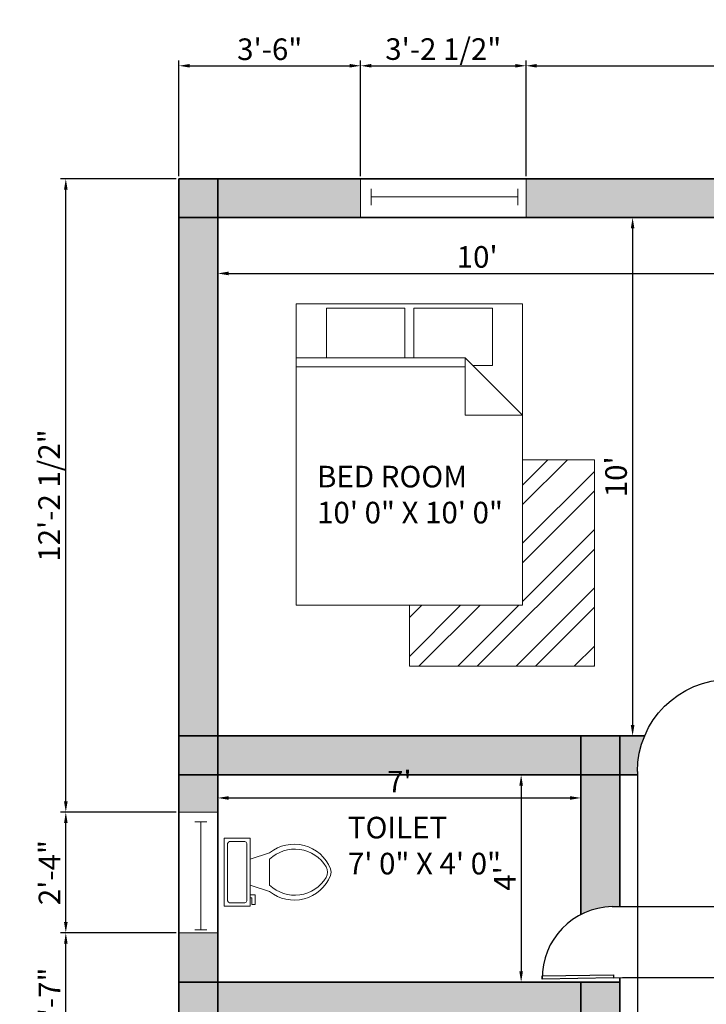
# Model space of a CAD drawing. Units: millimetres. Extents: x 2803 to 3393, y 965 to 1464.
# Tile 3 of 6: x 2803 to 2962, y 1236 to 1464. Entities that reach past the tile are written whole.
import ezdxf

# ---------------------------------------------------------------- set-up
doc = ezdxf.new("R2010")
doc.units = ezdxf.units.MM
for name, color, linetype, lineweight in [('A-ANNO-DIMS', 150, 'Continuous', 18), ('A-AREA-IDEN', 200, 'Continuous', 25), ('A-FLOR-FIXT', 70, 'Continuous', 18), ('A-FLOR-PATT', 3, 'Continuous', 13), ('A-WALL-PATT', 2, 'Continuous', 13), ('doors', 10, 'Continuous', 25), ('furniture', 70, 'Continuous', 18), ('walls', 2, 'Continuous', 35), ('windows', 30, 'Continuous', 20)]:
    doc.layers.add(name, color=color, linetype=linetype, lineweight=lineweight)
doc.styles.get("Standard").update_dxf_attribs({"font": 'arial.ttf'})
doc.dimstyles.new('ISO-25', dxfattribs={"dimtxt": 5, "dimasz": 2.5, "dimexe": 1.25, "dimexo": 0.625, "dimtad": 1, "dimdec": 0, "dimlunit": 3, "dimtxsty": 'Standard', "dimcen": 2.5, "dimadec": 0, "dimazin": 0, "dimtfac": 1, "dimtdec": 0, "dimtmove": 0, "dimatfit": 3, "dimfxl": 1, "dimarcsym": 0})

# ---------------------------------------------------------------- blocks, each defined once
blk = doc.blocks.new('*U2')
for p, q in [((0, 0), (0, -6)), ((40, 0), (40, -6))]:
    blk.add_line(p, q)
blk.add_lwpolyline([(0, 0), (0, 40), (1.75, 40), (1.75, 0)], close=True)
blk.add_arc((0, 0), 40, 0, 90)
blk = doc.blocks.new('*U6')
for p, q in [((0, 4), (0, 0)), ((36, 4), (36, 0)), ((0, 2), (36, 2))]:
    blk.add_line(p, q)
blk = doc.blocks.new('Bed - Queen')
for p, q in [((0, -80.00003), (0, 0)), ((0, 0), (59.99999, 0)), ((59.99999, 0), (59.99999, -80.00003)), ((7.99999, -1.2), (28.79998, -1.2)), ((7.99999, -14.4), (7.99999, -1.2)), ((28.79998, -1.2), (28.79998, -14.4)), ((31.19999, -1.2), (51.99999, -1.2)), ((31.19999, -14.4), (31.19999, -1.2)), ((51.99999, -1.2), (51.99999, -16.4)), ((0, -14.4), (44.8, -14.4)), ((59.99999, -29.6), (44.8, -14.4)), ((44.8, -14.4), (44.8, -29.6)), ((44.8, -16.8), (0, -16.8)), ((51.99999, -16.4), (46.79936, -16.4)), ((44.8, -29.6), (59.99999, -29.6)), ((59.99999, -80.00003), (0, -80.00003))]:
    blk.add_line(p, q)
blk = doc.blocks.new('Toilet - top')
for p, q in [((9.5, -6), (9.5, -2)), ((-10, -8.5), (-8, -8.5)), ((-10, -9.5), (-10, -8.5)), ((-8, -8.5), (-8, -8)), ((-7, -8), (-7, -9.5)), ((-4, -8), (-6, -14)), ((4, -8), (6, -14)), ((-7, -9.5), (-10, -9.5)), ((4, -14), (-4, -14))]:
    blk.add_line(p, q)
blk.add_lwpolyline([(10.5, -8), (10.5, 0), (-10.5, 0), (-10.5, -8)], close=True)
for points in [[(-9.5, -2), (-9.5, -6)], [(8.5, -1), (-8.5, -1)], [(-8.5, -7), (8.5, -7)]]:
    blk.add_lwpolyline(points)
for centre, radius, start, end in [((-8.62, -1.88), 0.884, 81.8699, 188.1301), ((8.62, -1.88), 0.884, 351.8699, 98.1301), ((-8.62, -6.12), 0.884, 171.8699, 278.1301), ((8.62, -6.12), 0.884, 261.8699, 8.1301), ((3.52, -21.58), 12.17, 141.4691, 247.9714), ((4.2, -21.82), 11.33, 136.3677, 238.9468), ((-3.52, -21.58), 12.17, 292.0284, 38.5307), ((-4.2, -21.82), 11.33, 301.053, 43.6321), ((0, -27.88), 4, 245.7318, 294.2682), ((0, -29), 4, 254.8605, 285.1395)]:
    blk.add_arc(centre, radius, start, end)
blk = doc.blocks.new('*D12')
at = {"layer": 'A-ANNO-DIMS', "color": 0, "lineweight": -2, "transparency": 16777216}
for p, q in [((2945.27, 1418.56), (2945.89, 1418.56)), ((2944.64, 1416.06), (2944.64, 1301.06)), ((2945.27, 1298.56), (2945.89, 1298.56))]:
    blk.add_line(p, q, dxfattribs=at)
at = {"layer": 'A-ANNO-DIMS', "color": 0, "transparency": 16777216}
for points in [[(2944.22, 1416.06), (2945.06, 1416.06), (2944.64, 1418.56)], [(2944.22, 1301.06), (2945.06, 1301.06), (2944.64, 1298.56)]]:
    blk.add_solid(points, dxfattribs=at)
at = {"layer": 'Defpoints', "color": 0, "transparency": 16777216}
for p in [(2944.64, 1418.56), (2944.64, 1298.56), (2944.64, 1298.56)]:
    blk.add_point(p, dxfattribs=at)
at = {"layer": 'A-ANNO-DIMS', "color": 0, "transparency": 16777216, "insert": (2941.46, 1358.56), "char_height": 5, "attachment_point": 5, "rotation": 90}
blk.add_mtext("10'", dxfattribs=at)
blk = doc.blocks.new('*D13')
at = {"layer": 'A-ANNO-DIMS', "color": 0, "lineweight": -2, "transparency": 16777216}
for p, q in [((2848.68, 1407.09), (2848.68, 1404.39)), ((2968.68, 1407.09), (2968.68, 1404.39)), ((2851.18, 1405.64), (2966.18, 1405.64))]:
    blk.add_line(p, q, dxfattribs=at)
at = {"layer": 'A-ANNO-DIMS', "color": 0, "transparency": 16777216}
for points in [[(2851.18, 1406.06), (2851.18, 1405.22), (2848.68, 1405.64)], [(2966.18, 1406.06), (2966.18, 1405.22), (2968.68, 1405.64)]]:
    blk.add_solid(points, dxfattribs=at)
at = {"layer": 'Defpoints', "color": 0, "transparency": 16777216}
for p in [(2848.68, 1407.71), (2968.68, 1407.71), (2968.68, 1405.64)]:
    blk.add_point(p, dxfattribs=at)
at = {"layer": 'A-ANNO-DIMS', "color": 0, "transparency": 16777216, "insert": (2908.68, 1408.82), "char_height": 5, "attachment_point": 5}
blk.add_mtext("10'", dxfattribs=at)
blk = doc.blocks.new('*D20')
at = {"layer": 'A-ANNO-DIMS', "color": 0, "lineweight": -2, "transparency": 16777216}
for p, q in [((2919.48, 1289.56), (2920.1, 1289.56)), ((2918.85, 1287.06), (2918.85, 1244.06)), ((2919.48, 1241.56), (2920.1, 1241.56))]:
    blk.add_line(p, q, dxfattribs=at)
at = {"layer": 'A-ANNO-DIMS', "color": 0, "transparency": 16777216}
for points in [[(2918.44, 1287.06), (2919.27, 1287.06), (2918.85, 1289.56)], [(2918.44, 1244.06), (2919.27, 1244.06), (2918.85, 1241.56)]]:
    blk.add_solid(points, dxfattribs=at)
at = {"layer": 'Defpoints', "color": 0, "transparency": 16777216}
for p in [(2918.85, 1289.56), (2918.85, 1241.56), (2918.85, 1241.56)]:
    blk.add_point(p, dxfattribs=at)
at = {"layer": 'A-ANNO-DIMS', "color": 0, "transparency": 16777216, "insert": (2915.73, 1265.56), "char_height": 5, "attachment_point": 5, "rotation": 90}
blk.add_mtext("4'", dxfattribs=at)
blk = doc.blocks.new('*D21')
at = {"layer": 'A-ANNO-DIMS', "color": 0, "lineweight": -2, "transparency": 16777216}
for p, q in [((2848.68, 1284.82), (2848.68, 1285.45)), ((2851.18, 1284.2), (2930.18, 1284.2)), ((2932.68, 1284.82), (2932.68, 1285.45))]:
    blk.add_line(p, q, dxfattribs=at)
at = {"layer": 'A-ANNO-DIMS', "color": 0, "transparency": 16777216}
for points in [[(2851.18, 1284.61), (2851.18, 1283.78), (2848.68, 1284.2)], [(2930.18, 1284.61), (2930.18, 1283.78), (2932.68, 1284.2)]]:
    blk.add_solid(points, dxfattribs=at)
at = {"layer": 'Defpoints', "color": 0, "transparency": 16777216}
for p in [(2848.68, 1284.2), (2932.68, 1284.2), (2932.68, 1284.2)]:
    blk.add_point(p, dxfattribs=at)
at = {"layer": 'A-ANNO-DIMS', "color": 0, "transparency": 16777216, "insert": (2890.68, 1287.32), "char_height": 5, "attachment_point": 5}
blk.add_mtext("7'", dxfattribs=at)
blk = doc.blocks.new('*D49')
at = {"layer": 'A-ANNO-DIMS', "color": 0, "lineweight": -2, "transparency": 16777216}
for p, q in [((2839.68, 1428.19), (2839.68, 1454.97)), ((2881.7, 1428.19), (2881.7, 1454.97)), ((2842.18, 1453.72), (2879.2, 1453.72))]:
    blk.add_line(p, q, dxfattribs=at)
at = {"layer": 'A-ANNO-DIMS', "color": 0, "transparency": 16777216}
for points in [[(2842.18, 1454.14), (2842.18, 1453.31), (2839.68, 1453.72)], [(2879.2, 1454.14), (2879.2, 1453.31), (2881.7, 1453.72)]]:
    blk.add_solid(points, dxfattribs=at)
at = {"layer": 'Defpoints', "color": 0, "transparency": 16777216}
for p in [(2881.7, 1453.72), (2839.68, 1427.56), (2881.7, 1427.56)]:
    blk.add_point(p, dxfattribs=at)
at = {"layer": 'A-ANNO-DIMS', "color": 0, "transparency": 16777216, "insert": (2860.69, 1456.9), "char_height": 5, "attachment_point": 5}
blk.add_mtext('3\'-6"', dxfattribs=at)
blk = doc.blocks.new('*D50')
at = {"layer": 'A-ANNO-DIMS', "color": 0, "lineweight": -2, "transparency": 16777216}
for p, q in [((2881.7, 1428.19), (2881.7, 1454.97)), ((2919.98, 1428.19), (2919.98, 1454.97)), ((2884.2, 1453.72), (2917.48, 1453.72))]:
    blk.add_line(p, q, dxfattribs=at)
at = {"layer": 'A-ANNO-DIMS', "color": 0, "transparency": 16777216}
for points in [[(2884.2, 1454.14), (2884.2, 1453.31), (2881.7, 1453.72)], [(2917.48, 1454.14), (2917.48, 1453.31), (2919.98, 1453.72)]]:
    blk.add_solid(points, dxfattribs=at)
at = {"layer": 'Defpoints', "color": 0, "transparency": 16777216}
for p in [(2919.98, 1453.72), (2881.7, 1427.56), (2919.98, 1427.56)]:
    blk.add_point(p, dxfattribs=at)
at = {"layer": 'A-ANNO-DIMS', "color": 0, "transparency": 16777216, "insert": (2900.84, 1456.94), "char_height": 5, "attachment_point": 5}
blk.add_mtext('3\'-2 1/2"', dxfattribs=at)
blk = doc.blocks.new('*D51')
at = {"layer": 'A-ANNO-DIMS', "color": 0, "lineweight": -2, "transparency": 16777216}
for p, q in [((2919.98, 1428.19), (2919.98, 1454.97)), ((3021.74, 1428.19), (3021.74, 1454.97)), ((2922.48, 1453.72), (3019.24, 1453.72))]:
    blk.add_line(p, q, dxfattribs=at)
at = {"layer": 'A-ANNO-DIMS', "color": 0, "transparency": 16777216}
for points in [[(2922.48, 1454.14), (2922.48, 1453.31), (2919.98, 1453.72)], [(3019.24, 1454.14), (3019.24, 1453.31), (3021.74, 1453.72)]]:
    blk.add_solid(points, dxfattribs=at)
at = {"layer": 'Defpoints', "color": 0, "transparency": 16777216}
for p in [(3021.74, 1453.72), (2919.98, 1427.56), (3021.74, 1427.56)]:
    blk.add_point(p, dxfattribs=at)
at = {"layer": 'A-ANNO-DIMS', "color": 0, "transparency": 16777216, "insert": (2970.86, 1456.9), "char_height": 5, "attachment_point": 5}
blk.add_mtext('8\'-6"', dxfattribs=at)
blk = doc.blocks.new('*D58')
at = {"layer": 'A-ANNO-DIMS', "color": 0, "lineweight": -2, "transparency": 16777216}
for p, q in [((2839.06, 1252.94), (2812.27, 1252.94)), ((2813.52, 1224.36), (2813.52, 1250.44)), ((2839.06, 1221.86), (2812.27, 1221.86))]:
    blk.add_line(p, q, dxfattribs=at)
at = {"layer": 'A-ANNO-DIMS', "color": 0, "transparency": 16777216}
for points in [[(2813.11, 1250.44), (2813.94, 1250.44), (2813.52, 1252.94)], [(2813.11, 1224.36), (2813.94, 1224.36), (2813.52, 1221.86)]]:
    blk.add_solid(points, dxfattribs=at)
at = {"layer": 'Defpoints', "color": 0, "transparency": 16777216}
for p in [(2813.52, 1252.94), (2839.68, 1252.94), (2839.68, 1221.86)]:
    blk.add_point(p, dxfattribs=at)
at = {"layer": 'A-ANNO-DIMS', "color": 0, "transparency": 16777216, "insert": (2810.39, 1237.4), "char_height": 5, "attachment_point": 5, "rotation": 90}
blk.add_mtext('2\'-7"', dxfattribs=at)
blk = doc.blocks.new('*D59')
at = {"layer": 'A-ANNO-DIMS', "color": 0, "lineweight": -2, "transparency": 16777216}
for p, q in [((2839.06, 1280.88), (2812.27, 1280.88)), ((2813.52, 1255.44), (2813.52, 1278.38)), ((2839.06, 1252.94), (2812.27, 1252.94))]:
    blk.add_line(p, q, dxfattribs=at)
at = {"layer": 'A-ANNO-DIMS', "color": 0, "transparency": 16777216}
for points in [[(2813.11, 1278.38), (2813.94, 1278.38), (2813.52, 1280.88)], [(2813.11, 1255.44), (2813.94, 1255.44), (2813.52, 1252.94)]]:
    blk.add_solid(points, dxfattribs=at)
at = {"layer": 'Defpoints', "color": 0, "transparency": 16777216}
for p in [(2813.52, 1280.88), (2839.68, 1280.88), (2839.68, 1252.94)]:
    blk.add_point(p, dxfattribs=at)
at = {"layer": 'A-ANNO-DIMS', "color": 0, "transparency": 16777216, "insert": (2810.39, 1266.91), "char_height": 5, "attachment_point": 5, "rotation": 90}
blk.add_mtext('2\'-4"', dxfattribs=at)
blk = doc.blocks.new('*D60')
at = {"layer": 'A-ANNO-DIMS', "color": 0, "lineweight": -2, "transparency": 16777216}
for p, q in [((2839.06, 1427.56), (2812.27, 1427.56)), ((2813.52, 1283.38), (2813.52, 1425.06)), ((2839.06, 1280.88), (2812.27, 1280.88))]:
    blk.add_line(p, q, dxfattribs=at)
at = {"layer": 'A-ANNO-DIMS', "color": 0, "transparency": 16777216}
for points in [[(2813.11, 1425.06), (2813.94, 1425.06), (2813.52, 1427.56)], [(2813.11, 1283.38), (2813.94, 1283.38), (2813.52, 1280.88)]]:
    blk.add_solid(points, dxfattribs=at)
at = {"layer": 'Defpoints', "color": 0, "transparency": 16777216}
for p in [(2813.52, 1427.56), (2839.68, 1427.56), (2839.68, 1280.88)]:
    blk.add_point(p, dxfattribs=at)
at = {"layer": 'A-ANNO-DIMS', "color": 0, "transparency": 16777216, "insert": (2810.31, 1354.22), "char_height": 5, "attachment_point": 5, "rotation": 90}
blk.add_mtext('12\'-2 1/2"', dxfattribs=at)
blk = doc.blocks.new('*D67')
at = {"layer": 'A-ANNO-DIMS', "color": 0, "lineweight": -2, "transparency": 16777216}
for p, q in [((2945.75, 1288.94), (2945.75, 968.15)), ((2967.14, 1288.94), (2967.14, 968.15)), ((2948.25, 969.4), (2964.64, 969.4)), ((2967.14, 969.4), (2995.36, 969.4))]:
    blk.add_line(p, q, dxfattribs=at)
at = {"layer": 'A-ANNO-DIMS', "color": 0, "transparency": 16777216}
for points in [[(2948.25, 969.82), (2948.25, 968.99), (2945.75, 969.4)], [(2964.64, 969.82), (2964.64, 968.99), (2967.14, 969.4)]]:
    blk.add_solid(points, dxfattribs=at)
at = {"layer": 'Defpoints', "color": 0, "transparency": 16777216}
for p in [(2945.75, 1289.56), (2967.14, 1289.56), (2967.14, 969.4)]:
    blk.add_point(p, dxfattribs=at)
at = {"layer": 'A-ANNO-DIMS', "color": 0, "transparency": 16777216, "insert": (2982.5, 972.61), "char_height": 5, "attachment_point": 5}
blk.add_mtext('1\'-9 1/2"', dxfattribs=at)
blk = doc.blocks.new('*D68')
at = {"layer": 'A-ANNO-DIMS', "color": 0, "lineweight": -2, "transparency": 16777216}
for p, q in [((3388.84, 1259.07), (3388.84, 1287.29)), ((2942.31, 1259.07), (3390.09, 1259.07)), ((3388.84, 1245.09), (3388.84, 1256.57)), ((2942.31, 1242.59), (3390.09, 1242.59))]:
    blk.add_line(p, q, dxfattribs=at)
at = {"layer": 'A-ANNO-DIMS', "color": 0, "transparency": 16777216}
for points in [[(3388.43, 1256.57), (3389.26, 1256.57), (3388.84, 1259.07)], [(3388.43, 1245.09), (3389.26, 1245.09), (3388.84, 1242.59)]]:
    blk.add_solid(points, dxfattribs=at)
at = {"layer": 'Defpoints', "color": 0, "transparency": 16777216}
for p in [(2941.68, 1259.07), (3388.84, 1259.07), (2941.68, 1242.59)]:
    blk.add_point(p, dxfattribs=at)
at = {"layer": 'A-ANNO-DIMS', "color": 0, "transparency": 16777216, "insert": (3385.63, 1274.43), "char_height": 5, "attachment_point": 5, "rotation": 90}
blk.add_mtext('1\'-4 1/2"', dxfattribs=at)
blk = doc.blocks.new('*D74')
at = {"layer": 'A-ANNO-DIMS', "color": 0, "lineweight": -2, "transparency": 16777216}
for p, q in [((3388.84, 1232.56), (3388.84, 1260.78)), ((2869.11, 1232.56), (3390.09, 1232.56)), ((3388.84, 1220.39), (3388.84, 1230.06)), ((2933.31, 1217.89), (3390.09, 1217.89))]:
    blk.add_line(p, q, dxfattribs=at)
at = {"layer": 'A-ANNO-DIMS', "color": 0, "transparency": 16777216}
for points in [[(3388.43, 1230.06), (3389.26, 1230.06), (3388.84, 1232.56)], [(3388.43, 1220.39), (3389.26, 1220.39), (3388.84, 1217.89)]]:
    blk.add_solid(points, dxfattribs=at)
at = {"layer": 'Defpoints', "color": 0, "transparency": 16777216}
for p in [(2868.49, 1232.56), (3388.84, 1232.56), (2932.68, 1217.89)]:
    blk.add_point(p, dxfattribs=at)
at = {"layer": 'A-ANNO-DIMS', "color": 0, "transparency": 16777216, "insert": (3385.63, 1247.92), "char_height": 5, "attachment_point": 5, "rotation": 90}
blk.add_mtext('1\'-2 1/2"', dxfattribs=at)

msp = doc.modelspace()

# ---------------------------------------------------------------- hatches: boundary and pattern name
at = {"layer": 'A-FLOR-PATT'}
h = msp.add_hatch(dxfattribs=at)
h.set_pattern_fill('ANSI32', color=256)
h.paths.add_polyline_path([(2935.82, 1362.49), (2919.19, 1362.49), (2919.19, 1328.83), (2893.01, 1328.83), (2893.01, 1314.7), (2935.82, 1314.7)])
h.paths.add_polyline_path([(2891.3, 1122.74), (2917.48, 1122.74), (2917.48, 1136.87), (2874.67, 1136.87), (2874.67, 1089.08), (2891.3, 1089.08)])
at = {"layer": 'A-WALL-PATT'}
h = msp.add_hatch(color=256, dxfattribs=at)
h.dxf.hatch_style = 1
h.paths.add_polyline_path([(2968.68, 1427.56), (2919.98, 1427.56), (2919.98, 1418.56), (2968.68, 1418.56)])
h.paths.add_polyline_path([(2977.68, 1427.56), (2968.68, 1427.56), (2968.68, 1418.56), (2977.68, 1418.56)])
h.paths.add_polyline_path([(2977.68, 1418.56), (2968.68, 1418.56), (2968.68, 1298.56), (2977.68, 1298.56)])
h.paths.add_polyline_path([(3021.74, 1427.56), (2977.68, 1427.56), (2977.68, 1418.56), (3021.74, 1418.56)])
h.paths.add_polyline_path([(2881.7, 1427.56), (2848.68, 1427.56), (2848.68, 1418.56), (2881.7, 1418.56)])
h.paths.add_polyline_path([(2848.68, 1427.56), (2839.68, 1427.56), (2839.68, 1418.56), (2848.68, 1418.56)])
h.paths.add_polyline_path([(2848.68, 1418.56), (2839.68, 1418.56), (2839.68, 1298.56), (2848.68, 1298.56)])
h.paths.add_polyline_path([(2932.68, 1298.56), (2848.68, 1298.56), (2848.68, 1289.56), (2932.68, 1289.56)])
h.paths.add_polyline_path([(2848.68, 1298.56), (2839.68, 1298.56), (2839.68, 1289.56), (2848.68, 1289.56)])
h.paths.add_polyline_path([(2848.68, 1289.56), (2839.68, 1289.56), (2839.68, 1280.88), (2848.68, 1280.88)])
h.paths.add_polyline_path([(2848.68, 1252.94), (2839.68, 1252.94), (2839.68, 1241.56), (2848.68, 1241.56)])
h.paths.add_polyline_path([(2848.68, 1241.56), (2839.68, 1241.56), (2839.68, 1232.56), (2848.68, 1232.56)])
h.paths.add_polyline_path([(2932.68, 1241.56), (2848.68, 1241.56), (2848.68, 1232.56), (2932.68, 1232.56)])
h.paths.add_polyline_path([(2941.68, 1241.56), (2932.68, 1241.56), (2932.68, 1232.56), (2941.68, 1232.56)])
h.paths.add_polyline_path([(2941.68, 1289.56), (2932.68, 1289.56), (2932.68, 1257.22, -0.114666), (2939.92, 1259.03), (2941.68, 1259.07)])
h.paths.add_polyline_path([(2941.68, 1298.56), (2932.68, 1298.56), (2932.68, 1289.56), (2941.68, 1289.56)])
h.paths.add_polyline_path([(2947.42, 1298.56), (2941.68, 1298.56), (2941.68, 1289.56), (2945.75, 1289.56), (2945.75, 1290.29, -0.099582)])
h.paths.add_polyline_path([(2977.68, 1298.56), (2968.68, 1298.56), (2968.68, 1289.56), (2977.68, 1289.56)])
h.paths.add_polyline_path([(3018.47, 1298.56), (2977.68, 1298.56), (2977.68, 1289.56), (3018.47, 1289.56)])
h.paths.add_polyline_path([(3097.68, 1298.56), (3067.31, 1298.56), (3067.31, 1289.56), (3097.68, 1289.56)])
h.paths.add_polyline_path([(3106.68, 1298.56), (3097.68, 1298.56), (3097.68, 1289.56), (3106.68, 1289.56)])
h.paths.add_polyline_path([(3200.68, 1298.56), (3106.68, 1298.56), (3106.68, 1289.56), (3200.68, 1289.56)])
h.paths.add_polyline_path([(3209.68, 1298.56), (3200.68, 1298.56), (3200.68, 1289.56), (3209.68, 1289.56)])
h.paths.add_polyline_path([(3209.68, 1289.56), (3200.68, 1289.56), (3200.68, 1270.22), (3209.68, 1270.22)])
h.paths.add_polyline_path([(3106.68, 1418.56), (3097.68, 1418.56), (3097.68, 1298.56), (3106.68, 1298.56)])
h.paths.add_polyline_path([(3106.68, 1427.56), (3097.68, 1427.56), (3097.68, 1418.56), (3106.68, 1418.56)])
h.paths.add_polyline_path([(3097.68, 1427.56), (3058.94, 1427.56), (3058.94, 1418.56), (3097.68, 1418.56)])
h.paths.add_polyline_path([(3353.68, 1427.56), (3106.68, 1427.56), (3106.68, 1418.56), (3353.68, 1418.56)])
h.paths.add_polyline_path([(3362.68, 1427.56), (3353.68, 1427.56), (3353.68, 1418.56), (3362.68, 1418.56)])
h.paths.add_polyline_path([(3362.68, 1418.56), (3353.68, 1418.56), (3353.68, 1064.56), (3362.68, 1064.56)])
h.paths.add_polyline_path([(3362.68, 1064.56), (3353.68, 1064.56), (3353.68, 1055.56), (3362.68, 1055.56)])
h.paths.add_polyline_path([(3362.68, 1055.56), (3353.68, 1055.56), (3353.68, 995.56), (3362.68, 995.56)])
h.paths.add_polyline_path([(3353.68, 1064.56), (3209.68, 1064.56), (3209.68, 1055.56), (3353.68, 1055.56)])
h.paths.add_polyline_path([(3200.68, 1064.56), (3106.68, 1064.56), (3106.68, 1055.56), (3200.68, 1055.56)])
h.paths.add_polyline_path([(3209.68, 1064.56), (3200.68, 1064.56), (3200.68, 1055.56), (3209.68, 1055.56)])
h.paths.add_polyline_path([(3209.68, 1229.61), (3200.68, 1229.61), (3200.68, 1064.56), (3209.68, 1064.56)])
h.paths.add_polyline_path([(3106.68, 1117.56), (3097.68, 1117.56), (3097.68, 1064.56), (3106.68, 1064.56)])
h.paths.add_polyline_path([(3106.68, 1126.56), (3097.68, 1126.56), (3097.68, 1117.56), (3106.68, 1117.56)])
h.paths.add_polyline_path([(3097.68, 1126.56), (3001.68, 1126.56), (3001.68, 1117.56), (3097.68, 1117.56)])
h.paths.add_polyline_path([(3001.68, 1165.56), (2992.68, 1165.56), (2992.68, 1126.56), (3001.68, 1126.56)])
h.paths.add_polyline_path([(3001.68, 1174.56), (2992.68, 1174.56), (2992.68, 1165.56), (3001.68, 1165.56)])
h.paths.add_polyline_path([(2992.68, 1174.56), (2986.69, 1174.56), (2986.69, 1165.56), (2992.68, 1165.56)])
h.paths.add_polyline_path([(3001.68, 1126.56), (2992.68, 1126.56), (2992.68, 1117.56), (3001.68, 1117.56)])
h.paths.add_polyline_path([(3001.68, 1117.56), (2992.68, 1117.56), (2992.68, 1112.21), (2994.15, 1112.23), (3001.68, 1112.37)])
h.paths.add_polyline_path([(3001.68, 1033.56), (2992.68, 1033.56), (2992.68, 1024.56), (3001.68, 1024.56)])
h.paths.add_polyline_path([(3001.68, 1097.58, -0.114732), (2994.45, 1095.76), (2992.68, 1095.73), (2992.68, 1033.56), (3001.68, 1033.56)])
h.paths.add_polyline_path([(3030.4, 1033.56), (3001.68, 1033.56), (3001.68, 1024.56), (3030.4, 1024.56)])
h.paths.add_polyline_path([(3097.68, 1033.56), (3060.2, 1033.56), (3060.2, 1024.56), (3097.68, 1024.56)])
h.paths.add_polyline_path([(3106.68, 1033.56), (3097.68, 1033.56), (3097.68, 1024.56), (3106.68, 1024.56)])
h.paths.add_polyline_path([(3106.68, 1055.56), (3097.68, 1055.56), (3097.68, 1033.56), (3106.68, 1033.56)])
h.paths.add_polyline_path([(3106.68, 1064.56), (3097.68, 1064.56), (3097.68, 1055.56), (3106.68, 1055.56)])
h.paths.add_polyline_path([(2992.68, 1033.56), (2848.68, 1033.56), (2848.68, 1024.56), (2992.68, 1024.56)])
h.paths.add_polyline_path([(2848.68, 1033.56), (2839.68, 1033.56), (2839.68, 1024.56), (2848.68, 1024.56)])
h.paths.add_polyline_path([(2848.68, 1070.54), (2839.68, 1070.54), (2839.68, 1033.56), (2848.68, 1033.56)])
h.paths.add_polyline_path([(2848.68, 1165.56), (2839.68, 1165.56), (2839.68, 1114.52), (2848.68, 1114.52)])
h.paths.add_polyline_path([(2848.68, 1174.56), (2839.68, 1174.56), (2839.68, 1165.56), (2848.68, 1165.56)])
h.paths.add_polyline_path([(2932.68, 1174.56), (2848.68, 1174.56), (2848.68, 1165.56), (2932.68, 1165.56)])
h.paths.add_polyline_path([(2941.68, 1174.56), (2932.68, 1174.56), (2932.68, 1165.56), (2941.68, 1165.56)])
h.paths.add_polyline_path([(2965.38, 1174.56), (2941.68, 1174.56), (2941.68, 1165.56), (2968.2, 1165.56, -0.111634)])
h.paths.add_polyline_path([(2848.68, 1193.13), (2839.68, 1193.13), (2839.68, 1174.56), (2848.68, 1174.56)])
h.paths.add_polyline_path([(2848.68, 1232.56), (2839.68, 1232.56), (2839.68, 1221.86), (2848.68, 1221.86)])
h.paths.add_polyline_path([(2941.68, 1232.56), (2932.68, 1232.56), (2932.68, 1191.24, -0.132111), (2940.91, 1193.6), (2941.68, 1193.62)])
h.paths.add_polyline_path([(3106.68, 1262.96), (3105.94, 1262.96, -0.099353), (3097.68, 1264.61), (3097.68, 1126.56), (3106.68, 1126.56)])

# ---------------------------------------------------------------- linework, layer by layer
at = {"layer": 'furniture'}
for p, q in [((2919.19, 1362.49), (2935.82, 1362.49)), ((2935.82, 1362.49), (2935.82, 1314.7)), ((2893.01, 1314.7), (2893.01, 1328.83)), ((2935.82, 1314.7), (2893.01, 1314.7))]:
    msp.add_line(p, q, dxfattribs=at)
at = {"layer": 'walls'}
for p, q in [((2839.68, 1427.56), (2839.68, 1024.56)), ((2839.68, 1427.56), (3362.68, 1427.56)), ((2848.68, 1427.56), (2848.68, 1024.56)), ((2839.68, 1418.56), (3362.68, 1418.56)), ((2839.68, 1298.56), (2947.42, 1298.56)), ((2932.68, 1298.56), (2932.68, 1257.22)), ((2941.68, 1298.56), (2941.68, 1259.07)), ((2839.68, 1289.56), (2945.75, 1289.56)), ((2941.68, 1242.59), (2941.68, 1193.62)), ((2839.68, 1241.56), (2941.68, 1241.56)), ((2932.68, 1241.56), (2932.68, 1191.24))]:
    msp.add_line(p, q, dxfattribs=at)
at = {"layer": 'windows'}
for p, q in [((2881.7, 1427.56), (2881.7, 1418.56)), ((2919.98, 1427.56), (2919.98, 1418.56)), ((2848.68, 1280.88), (2839.68, 1280.88)), ((2848.68, 1252.94), (2839.68, 1252.94))]:
    msp.add_line(p, q, dxfattribs=at)

# ---------------------------------------------------------------- block references
at = {"layer": 'A-FLOR-FIXT', "xscale": 0.7483515901231887, "yscale": 0.7483515901231887, "zscale": 0.7483515901231887, "rotation": 89.99999999999999}
msp.add_blockref('Toilet - top', (2850.18, 1267.02), dxfattribs=at)
at = {"layer": 'doors', "xscale": -0.534749261424752, "yscale": 0.534749261424752, "zscale": 0.534749261424752}
msp.add_blockref('*U2', (2967.14, 1290.29), dxfattribs=at)
at = {"layer": 'doors', "xscale": 0.4118610338034785, "yscale": 0.4118610338034785, "zscale": 0.4118610338034785, "rotation": 91.02414730254725}
msp.add_blockref('*U2', (2940.21, 1242.56), dxfattribs=at)
at = {"layer": 'furniture', "xscale": 0.8725478545565646, "yscale": 0.8725478545565646, "zscale": 0.8725478545565646}
msp.add_blockref('Bed - Queen', (2866.84, 1398.64), dxfattribs=at)
at = {"layer": 'windows', "xscale": 0.9425308196764994, "yscale": 0.9425308196764994, "zscale": 0.9425308196764994}
msp.add_blockref('*U6', (2884.15, 1421.48), dxfattribs=at)
at = {"layer": 'windows', "xscale": 0.6948136988430634, "yscale": 0.6948136988430634, "zscale": 0.6948136988430634, "rotation": 90}
msp.add_blockref('*U6', (2846.14, 1253.66), dxfattribs=at)

# ---------------------------------------------------------------- texts
at = {"layer": 'A-AREA-IDEN', "char_height": 5, "attachment_point": 1}
for s, width, insert in [('BED ROOM \\P10\' 0" X 10\' 0"', 44.718, (2871.65, 1361.1)), ('TOILET \\P7\' 0" X 4\' 0"', 45.557, (2878.78, 1279.83))]:
    msp.add_mtext_dynamic_manual_height_columns(s, width=width, gutter_width=12.5, heights=[0], dxfattribs=dict(at, insert=insert))

# ---------------------------------------------------------------- dimensions: what is measured, and where the dimension line sits
at = {"layer": 'A-ANNO-DIMS'}
for base, p1, p2, override, picture, middle in [((2919.98, 1453.72), (2881.7, 1427.56), (2919.98, 1427.56), {"dimdec": 1, "dimlfac": 1, "dimrnd": 0, "dimzin": 1, "dimdsep": 46, "dimlunit": 4, "dimfrac": 2}, '*D50', (2900.84, 1456.94)), ((2881.7, 1453.72), (2839.68, 1427.56), (2881.7, 1427.56), {"dimdec": 1, "dimlfac": 1, "dimrnd": 0, "dimzin": 1, "dimdsep": 46, "dimlunit": 4, "dimfrac": 2}, '*D49', (2860.69, 1456.9)), ((3021.74, 1453.72), (2919.98, 1427.56), (3021.74, 1427.56), {"dimdec": 1, "dimlfac": 1, "dimrnd": 0, "dimzin": 1, "dimdsep": 46, "dimlunit": 4, "dimfrac": 2}, '*D51', (2970.86, 1456.9)), ((2968.68, 1405.64), (2848.68, 1407.71), (2968.68, 1407.71), {"dimclrd": 0, "dimclre": 0, "dimclrt": 0}, '*D13', (2908.68, 1408.82)), ((2932.68, 1284.2), (2848.68, 1284.2), (2932.68, 1284.2), {"dimclrd": 0, "dimclre": 0, "dimclrt": 0}, '*D21', (2890.68, 1287.32)), ((2967.14, 969.4), (2945.75, 1289.56), (2967.14, 1289.56), {"dimdec": 1, "dimlfac": 1, "dimrnd": 0, "dimzin": 1, "dimdsep": 46, "dimlunit": 4, "dimfrac": 2}, '*D67', (2982.5, 972.61))]:
    dim = msp.add_linear_dim(base=base, p1=p1, p2=p2, dimstyle='ISO-25', override=override, dxfattribs=at)
    dim.commit()
    dim.dimension.update_dxf_attribs({"geometry": picture, "text_midpoint": middle})
for base, p1, p2, override, picture, middle in [((2813.52, 1427.56), (2839.68, 1280.88), (2839.68, 1427.56), {"dimdec": 1, "dimlfac": 1, "dimrnd": 0, "dimzin": 1, "dimdsep": 46, "dimlunit": 4, "dimfrac": 2}, '*D60', (2810.31, 1354.22)), ((2944.64, 1298.56), (2944.64, 1418.56), (2944.64, 1298.56), {"dimclrd": 0, "dimclre": 0, "dimclrt": 0}, '*D12', (2941.46, 1358.56)), ((2918.85, 1241.56), (2918.85, 1289.56), (2918.85, 1241.56), {"dimclrd": 0, "dimclre": 0, "dimclrt": 0}, '*D20', (2915.73, 1265.56)), ((3388.84, 1259.07), (2941.68, 1242.59), (2941.68, 1259.07), {"dimdec": 1, "dimlfac": 1, "dimrnd": 0, "dimzin": 1, "dimdsep": 46, "dimlunit": 4, "dimfrac": 2}, '*D68', (3385.63, 1274.43)), ((2813.52, 1280.88), (2839.68, 1252.94), (2839.68, 1280.88), {"dimdec": 1, "dimlfac": 1, "dimrnd": 0, "dimzin": 1, "dimdsep": 46, "dimlunit": 4, "dimfrac": 2}, '*D59', (2810.39, 1266.91)), ((3388.84, 1232.56), (2932.68, 1217.89), (2868.49, 1232.56), {"dimdec": 1, "dimlfac": 1, "dimrnd": 0, "dimzin": 1, "dimdsep": 46, "dimlunit": 4, "dimfrac": 2}, '*D74', (3385.63, 1247.92)), ((2813.52, 1252.94), (2839.68, 1221.86), (2839.68, 1252.94), {"dimdec": 1, "dimlfac": 1, "dimrnd": 0, "dimzin": 1, "dimdsep": 46, "dimlunit": 4, "dimfrac": 2}, '*D58', (2810.39, 1237.4))]:
    dim = msp.add_linear_dim(base=base, p1=p1, p2=p2, angle=90, dimstyle='ISO-25', override=override, dxfattribs=at)
    dim.commit()
    dim.dimension.update_dxf_attribs({"geometry": picture, "text_midpoint": middle})

doc.saveas('drawing.dxf')
